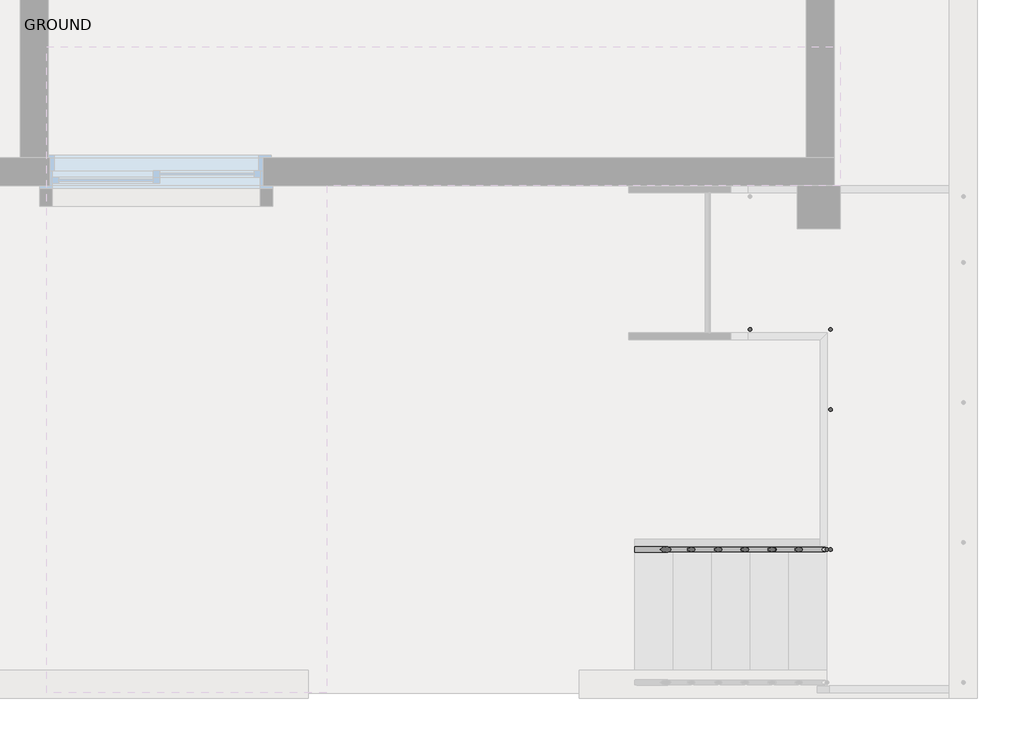
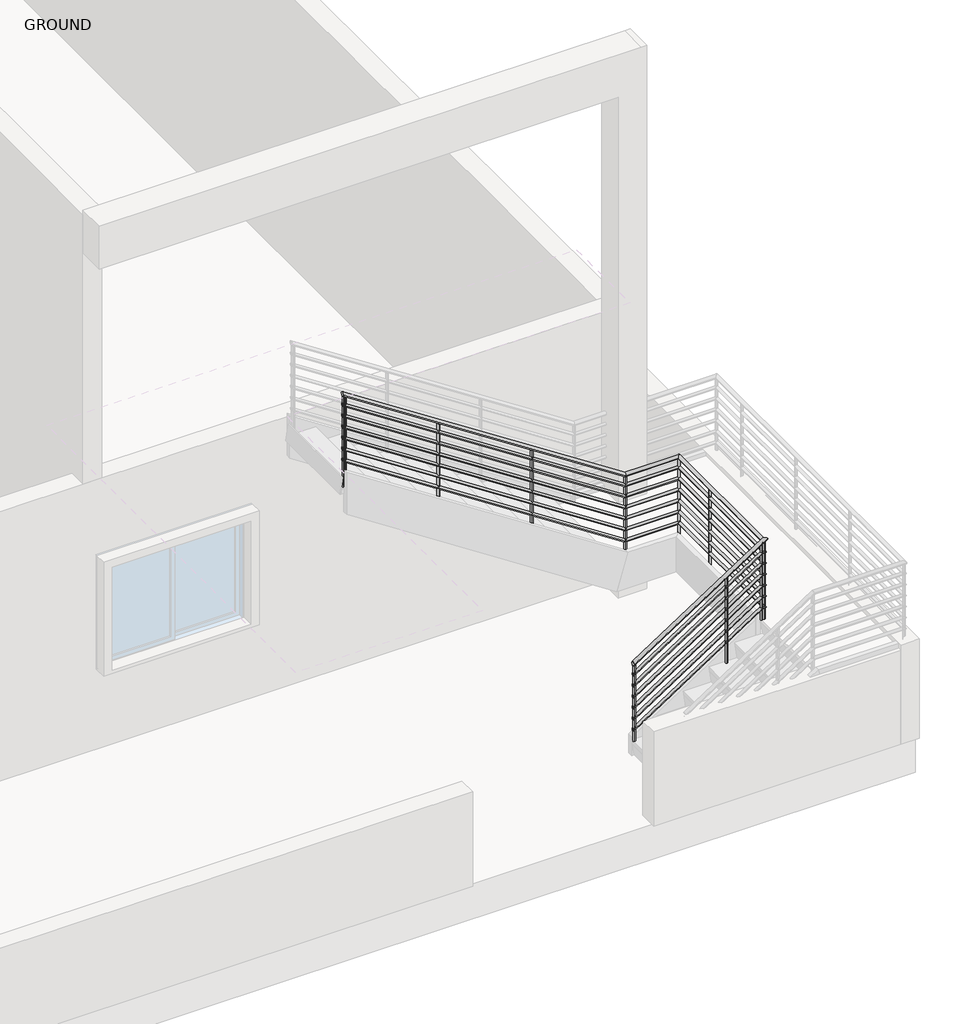
# One storey, part 3 of 4: 1 railing.
"""IFC4 building model written with IfcOpenShell, lengths in millimetres."""

from ifc_helpers import new_model, si_unit, point, frame, frame_2d, origin, place, context, project, spatial, circle_curve, ellipse_curve, trimmed, segment, composite_curve, outline, extrude, element, save
from ifc_brep_helpers import plane_surface, cylinder_surface, advanced_brep

model = new_model("IFC4")

# Units and contexts
model_context = context("Model", 3, world=origin())
ifc_project = project(units=[si_unit("LENGTHUNIT", "METRE", prefix="MILLI")], contexts=[model_context])

# Site, building, storey
site = spatial("IfcSite", under=ifc_project)
building = spatial("IfcBuilding", under=site)
storey = spatial("IfcBuildingStorey", under=building, Name="GROUND", Elevation=0.0)

# Railing
placement = place(None, origin())
element("IfcRailing", 1, ObjectType="900mm Pipe", at=placement, inside=storey, context=model_context, shape_type="SolidModel", body=[
    advanced_brep(
    [(11825.7864069, -2579.127917, 1055.4188073), (11825.7864069, -2539.127917, 1055.4188073), (13253.8631757, -2579.127917, 1986.4943135), (13220.3557578, -2539.127917, 1964.6481938)],
    [
        (0, 1, ellipse_curve(frame((11825.7864069, -2559.127917, 1055.4188073), z_axis=(-1.0, 0.0, 0.0), x_axis=(0.0, 0.0, -1.0)), 23.8753103, 20.0)),
        (1, 0, ellipse_curve(frame((11825.7864069, -2559.127917, 1055.4188073), z_axis=(-1.0, 0.0, 0.0), x_axis=(0.0, 0.0, -1.0)), 23.8753103, 20.0)),
        (2, 3, ellipse_curve(frame((13237.1094668, -2559.127917, 1975.5712536), z_axis=(0.592333060098466, 0.7071067811865425, 0.3861884849583095), x_axis=(-0.5923330600984512, 0.7071067811865527, -0.3861884849583129)), 28.2842712, 20.0)),
        (3, 2, ellipse_curve(frame((13237.1094668, -2559.127917, 1975.5712536), z_axis=(0.592333060098466, 0.7071067811865425, 0.3861884849583095), x_axis=(-0.5923330600984512, 0.7071067811865527, -0.3861884849583129)), 28.2842712, 20.0)),
        (0, 2),
        (3, 1),
    ],
    [
        plane_surface(frame((11825.7864069, -2559.127917, 1079.2941176), z_axis=(-1.0, 0.0, 0.0), x_axis=(0.0, 1.0, 0.0))),
        plane_surface(frame((13226.1864069, -2559.127917, 1992.3249626), z_axis=(0.592333060098466, 0.7071067811865425, 0.3861884849583095), x_axis=(0.8056932083084648, -0.5198538590091285, -0.2839197410518156))),
        cylinder_surface(frame((11836.7094668, -2559.127917, 1062.5404087), z_axis=(-0.8376854470331978, 0.0, -0.5461529930603618), x_axis=(0.0, 1.0, 0.0)), 20.0),
    ],
    [
        (0, [[1, 2]]),
        (1, [[3, 4]]),
        (2, [[-1, 5, -4, 6]]),
        (2, [[-2, -6, -3, -5]]),
    ],
),
    advanced_brep(
    [(13246.1864069, -2564.9585661, 1955.7647059), (13206.1864069, -2531.4511482, 1955.7647059), (13246.1864069, -966.5101069, 1955.7647059), (13206.1864069, -1006.5101069, 1955.7647059), (12644.8424844, -966.5101069, 1955.7647059), (12644.8424844, -1006.5101069, 1955.7647059), (9625.7864069, -966.5101069, 3924.1246897), (9625.7864069, -1006.5101069, 3924.1246897)],
    [
        (0, 1, ellipse_curve(frame((13226.1864069, -2548.2048572, 1955.7647059), z_axis=(-0.592333060098466, -0.7071067811865425, -0.3861884849583095), x_axis=(0.5923330600984515, -0.7071067811865525, 0.3861884849583132)), 28.2842712, 20.0)),
        (1, 0, ellipse_curve(frame((13226.1864069, -2548.2048572, 1955.7647059), z_axis=(-0.592333060098466, -0.7071067811865425, -0.3861884849583095), x_axis=(0.5923330600984515, -0.7071067811865525, 0.3861884849583132)), 28.2842712, 20.0)),
        (0, 2),
        (2, 3, ellipse_curve(frame((13226.1864069, -986.5101069, 1955.7647059), z_axis=(0.7071067811865414, -0.7071067811865537, 0.0), x_axis=(-0.7071067811865537, -0.7071067811865414, 0.0)), 28.2842712, 20.0)),
        (3, 1),
        (3, 2, ellipse_curve(frame((13226.1864069, -986.5101069, 1955.7647059), z_axis=(0.7071067811865414, -0.7071067811865537, 0.0), x_axis=(-0.7071067811865537, -0.7071067811865414, 0.0)), 28.2842712, 20.0)),
        (2, 4),
        (4, 5, ellipse_curve(frame((12644.8424844, -986.5101069, 1955.7647059), z_axis=(0.958562842758157, 0.0, -0.28488116203673575), x_axis=(0.2848811620367357, 0.0, 0.958562842758157)), 20.8645684, 20.0)),
        (5, 3),
        (5, 4, ellipse_curve(frame((12644.8424844, -986.5101069, 1955.7647059), z_axis=(0.958562842758157, 0.0, -0.28488116203673575), x_axis=(0.2848811620367357, 0.0, 0.958562842758157)), 20.8645684, 20.0)),
        (6, 7, ellipse_curve(frame((9625.7864069, -986.5101069, 3924.1246897), z_axis=(-1.0, 0.0, 0.0), x_axis=(0.0, 0.0, -1.0)), 23.8753103, 20.0)),
        (7, 6, ellipse_curve(frame((9625.7864069, -986.5101069, 3924.1246897), z_axis=(-1.0, 0.0, 0.0), x_axis=(0.0, 0.0, -1.0)), 23.8753103, 20.0)),
        (4, 6),
        (7, 5),
    ],
    [
        plane_surface(frame((13226.1864069, -2559.127917, 1975.7647059), z_axis=(-0.592333060098466, -0.7071067811865425, -0.3861884849583095), x_axis=(0.8056932083084648, -0.5198538590091285, -0.2839197410518156))),
        cylinder_surface(frame((13226.1864069, -2559.127917, 1955.7647059), z_axis=(0.0, -1.0, 0.0), x_axis=(-1.0, 0.0, 0.0)), 20.0),
        cylinder_surface(frame((13226.1864069, -986.5101069, 1955.7647059), z_axis=(1.0, 0.0, 0.0), x_axis=(0.0, -1.0, 0.0)), 20.0),
        plane_surface(frame((9625.7864069, -986.5101069, 3948.0), z_axis=(-1.0, 0.0, 0.0), x_axis=(0.0, -1.0, 0.0))),
        cylinder_surface(frame((12639.863347, -986.5101069, 1959.0109969), z_axis=(0.8376854470331982, 0.0, -0.5461529930603611), x_axis=(0.0, -1.0, 0.0)), 20.0),
    ],
    [
        (0, [[1, 2]]),
        (1, [[-1, 3, 4, 5]]),
        (1, [[-2, -5, 6, -3]]),
        (2, [[-4, 7, 8, 9]]),
        (2, [[-6, -9, 10, -7]]),
        (3, [[11, 12]]),
        (4, [[-8, 13, -12, 14]]),
        (4, [[-10, -14, -11, -13]]),
    ],
),
    advanced_brep(
    [(11825.7864069, -2574.127917, 936.3876349), (11825.7864069, -2544.127917, 936.3876349), (13205.2443488, -2574.127917, 1835.7647059), (13205.2443488, -2544.127917, 1835.7647059), (13241.1864069, -2574.127917, 1835.7647059), (13211.1864069, -2544.127917, 1835.7647059), (13241.1864069, -971.5101069, 1835.7647059), (13211.1864069, -1001.5101069, 1835.7647059), (12646.328465, -971.5101069, 1835.7647059), (12646.328465, -1001.5101069, 1835.7647059), (9625.7864069, -971.5101069, 3805.0935173), (9625.7864069, -1001.5101069, 3805.0935173)],
    [
        (0, 1, ellipse_curve(frame((11825.7864069, -2559.127917, 936.3876349), z_axis=(-1.0, 0.0, 0.0), x_axis=(0.0, 0.0, -1.0)), 17.9064827, 15.0)),
        (1, 0, ellipse_curve(frame((11825.7864069, -2559.127917, 936.3876349), z_axis=(-1.0, 0.0, 0.0), x_axis=(0.0, 0.0, -1.0)), 17.9064827, 15.0)),
        (0, 2),
        (2, 3, ellipse_curve(frame((13205.2443488, -2559.127917, 1835.7647059), z_axis=(-0.9585628427581571, 0.0, -0.2848811620367355), x_axis=(0.2848811620367357, 0.0, -0.9585628427581568)), 15.6484263, 15.0)),
        (3, 1),
        (3, 2, ellipse_curve(frame((13205.2443488, -2559.127917, 1835.7647059), z_axis=(-0.9585628427581571, 0.0, -0.2848811620367355), x_axis=(0.2848811620367357, 0.0, -0.9585628427581568)), 15.6484263, 15.0)),
        (2, 4),
        (4, 5, ellipse_curve(frame((13226.1864069, -2559.127917, 1835.7647059), z_axis=(-0.7071067811865537, -0.7071067811865414, 0.0), x_axis=(-0.7071067811865414, 0.7071067811865537, 0.0)), 21.2132034, 15.0)),
        (5, 3),
        (5, 4, ellipse_curve(frame((13226.1864069, -2559.127917, 1835.7647059), z_axis=(-0.7071067811865537, -0.7071067811865414, 0.0), x_axis=(-0.7071067811865414, 0.7071067811865537, 0.0)), 21.2132034, 15.0)),
        (4, 6),
        (6, 7, ellipse_curve(frame((13226.1864069, -986.5101069, 1835.7647059), z_axis=(0.7071067811865414, -0.7071067811865537, 0.0), x_axis=(-0.7071067811865538, -0.7071067811865414, 0.0)), 21.2132034, 15.0)),
        (7, 5),
        (7, 6, ellipse_curve(frame((13226.1864069, -986.5101069, 1835.7647059), z_axis=(0.7071067811865414, -0.7071067811865537, 0.0), x_axis=(-0.7071067811865538, -0.7071067811865414, 0.0)), 21.2132034, 15.0)),
        (6, 8),
        (8, 9, ellipse_curve(frame((12646.328465, -986.5101069, 1835.7647059), z_axis=(0.958562842758157, 0.0, -0.2848811620367359), x_axis=(0.28488116203673564, 0.0, 0.958562842758157)), 15.6484263, 15.0)),
        (9, 7),
        (9, 8, ellipse_curve(frame((12646.328465, -986.5101069, 1835.7647059), z_axis=(0.958562842758157, 0.0, -0.2848811620367359), x_axis=(0.28488116203673564, 0.0, 0.958562842758157)), 15.6484263, 15.0)),
        (10, 11, ellipse_curve(frame((9625.7864069, -986.5101069, 3805.0935173), z_axis=(-1.0, 0.0, 0.0), x_axis=(0.0, 0.0, -1.0)), 17.9064827, 15.0)),
        (11, 10, ellipse_curve(frame((9625.7864069, -986.5101069, 3805.0935173), z_axis=(-1.0, 0.0, 0.0), x_axis=(0.0, 0.0, -1.0)), 17.9064827, 15.0)),
        (8, 10),
        (11, 9),
    ],
    [
        plane_surface(frame((11825.7864069, -2559.127917, 954.2941176), z_axis=(-1.0, 0.0, 0.0), x_axis=(0.0, 1.0, 0.0))),
        cylinder_surface(frame((11833.9787018, -2559.127917, 941.7288359), z_axis=(-0.8376854470331986, 0.0, -0.5461529930603606), x_axis=(0.0, 1.0, 0.0)), 15.0),
        cylinder_surface(frame((13200.7864069, -2559.127917, 1835.7647059), z_axis=(-1.0, 0.0, 0.0), x_axis=(0.0, 1.0, 0.0)), 15.0),
        cylinder_surface(frame((13226.1864069, -2559.127917, 1835.7647059), z_axis=(0.0, -1.0, 0.0), x_axis=(-1.0, 0.0, 0.0)), 15.0),
        cylinder_surface(frame((13226.1864069, -986.5101069, 1835.7647059), z_axis=(1.0, 0.0, 0.0), x_axis=(0.0, -1.0, 0.0)), 15.0),
        plane_surface(frame((9625.7864069, -986.5101069, 3823.0), z_axis=(-1.0, 0.0, 0.0), x_axis=(0.0, -1.0, 0.0))),
        cylinder_surface(frame((12642.594112, -986.5101069, 1838.1994242), z_axis=(0.8376854470331982, 0.0, -0.5461529930603612), x_axis=(0.0, -1.0, 0.0)), 15.0),
    ],
    [
        (0, [[1, 2]]),
        (1, [[-1, 3, 4, 5]]),
        (1, [[-2, -5, 6, -3]]),
        (2, [[-4, 7, 8, 9]]),
        (2, [[-6, -9, 10, -7]]),
        (3, [[-8, 11, 12, 13]]),
        (3, [[-10, -13, 14, -11]]),
        (4, [[-12, 15, 16, 17]]),
        (4, [[-14, -17, 18, -15]]),
        (5, [[19, 20]]),
        (6, [[-16, 21, -20, 22]]),
        (6, [[-18, -22, -19, -21]]),
    ],
),
    advanced_brep(
    [(11825.7864069, -2574.127917, 811.3876349), (11825.7864069, -2544.127917, 811.3876349), (13205.2443488, -2574.127917, 1710.7647059), (13205.2443488, -2544.127917, 1710.7647059), (13241.1864069, -2574.127917, 1710.7647059), (13211.1864069, -2544.127917, 1710.7647059), (13241.1864069, -971.5101069, 1710.7647059), (13211.1864069, -1001.5101069, 1710.7647059), (12646.328465, -971.5101069, 1710.7647059), (12646.328465, -1001.5101069, 1710.7647059), (9625.7864069, -971.5101069, 3680.0935173), (9625.7864069, -1001.5101069, 3680.0935173)],
    [
        (0, 1, ellipse_curve(frame((11825.7864069, -2559.127917, 811.3876349), z_axis=(-1.0, 0.0, 0.0), x_axis=(0.0, 0.0, -1.0)), 17.9064827, 15.0)),
        (1, 0, ellipse_curve(frame((11825.7864069, -2559.127917, 811.3876349), z_axis=(-1.0, 0.0, 0.0), x_axis=(0.0, 0.0, -1.0)), 17.9064827, 15.0)),
        (0, 2),
        (2, 3, ellipse_curve(frame((13205.2443488, -2559.127917, 1710.7647059), z_axis=(-0.9585628427581571, 0.0, -0.2848811620367356), x_axis=(0.2848811620367359, 0.0, -0.958562842758157)), 15.6484263, 15.0)),
        (3, 1),
        (3, 2, ellipse_curve(frame((13205.2443488, -2559.127917, 1710.7647059), z_axis=(-0.9585628427581571, 0.0, -0.2848811620367356), x_axis=(0.2848811620367359, 0.0, -0.958562842758157)), 15.6484263, 15.0)),
        (2, 4),
        (4, 5, ellipse_curve(frame((13226.1864069, -2559.127917, 1710.7647059), z_axis=(-0.7071067811865537, -0.7071067811865414, 0.0), x_axis=(-0.7071067811865414, 0.7071067811865537, 0.0)), 21.2132034, 15.0)),
        (5, 3),
        (5, 4, ellipse_curve(frame((13226.1864069, -2559.127917, 1710.7647059), z_axis=(-0.7071067811865537, -0.7071067811865414, 0.0), x_axis=(-0.7071067811865414, 0.7071067811865537, 0.0)), 21.2132034, 15.0)),
        (4, 6),
        (6, 7, ellipse_curve(frame((13226.1864069, -986.5101069, 1710.7647059), z_axis=(0.7071067811865414, -0.7071067811865537, 0.0), x_axis=(-0.7071067811865538, -0.7071067811865414, 0.0)), 21.2132034, 15.0)),
        (7, 5),
        (7, 6, ellipse_curve(frame((13226.1864069, -986.5101069, 1710.7647059), z_axis=(0.7071067811865414, -0.7071067811865537, 0.0), x_axis=(-0.7071067811865538, -0.7071067811865414, 0.0)), 21.2132034, 15.0)),
        (6, 8),
        (8, 9, ellipse_curve(frame((12646.328465, -986.5101069, 1710.7647059), z_axis=(0.958562842758157, 0.0, -0.28488116203673575), x_axis=(0.2848811620367357, 0.0, 0.958562842758157)), 15.6484263, 15.0)),
        (9, 7),
        (9, 8, ellipse_curve(frame((12646.328465, -986.5101069, 1710.7647059), z_axis=(0.958562842758157, 0.0, -0.28488116203673575), x_axis=(0.2848811620367357, 0.0, 0.958562842758157)), 15.6484263, 15.0)),
        (10, 11, ellipse_curve(frame((9625.7864069, -986.5101069, 3680.0935173), z_axis=(-1.0, 0.0, 0.0), x_axis=(0.0, 0.0, -1.0)), 17.9064827, 15.0)),
        (11, 10, ellipse_curve(frame((9625.7864069, -986.5101069, 3680.0935173), z_axis=(-1.0, 0.0, 0.0), x_axis=(0.0, 0.0, -1.0)), 17.9064827, 15.0)),
        (8, 10),
        (11, 9),
    ],
    [
        plane_surface(frame((11825.7864069, -2559.127917, 829.2941176), z_axis=(-1.0, 0.0, 0.0), x_axis=(0.0, 1.0, 0.0))),
        cylinder_surface(frame((11833.9787018, -2559.127917, 816.7288359), z_axis=(-0.8376854470331985, 0.0, -0.5461529930603608), x_axis=(0.0, 1.0, 0.0)), 15.0),
        cylinder_surface(frame((13200.7864069, -2559.127917, 1710.7647059), z_axis=(-1.0, 0.0, 0.0), x_axis=(0.0, 1.0, 0.0)), 15.0),
        cylinder_surface(frame((13226.1864069, -2559.127917, 1710.7647059), z_axis=(0.0, -1.0, 0.0), x_axis=(-1.0, 0.0, 0.0)), 15.0),
        cylinder_surface(frame((13226.1864069, -986.5101069, 1710.7647059), z_axis=(1.0, 0.0, 0.0), x_axis=(0.0, -1.0, 0.0)), 15.0),
        plane_surface(frame((9625.7864069, -986.5101069, 3698.0), z_axis=(-1.0, 0.0, 0.0), x_axis=(0.0, -1.0, 0.0))),
        cylinder_surface(frame((12642.594112, -986.5101069, 1713.1994242), z_axis=(0.8376854470331982, 0.0, -0.5461529930603611), x_axis=(0.0, -1.0, 0.0)), 15.0),
    ],
    [
        (0, [[1, 2]]),
        (1, [[-1, 3, 4, 5]]),
        (1, [[-2, -5, 6, -3]]),
        (2, [[-4, 7, 8, 9]]),
        (2, [[-6, -9, 10, -7]]),
        (3, [[-8, 11, 12, 13]]),
        (3, [[-10, -13, 14, -11]]),
        (4, [[-12, 15, 16, 17]]),
        (4, [[-14, -17, 18, -15]]),
        (5, [[19, 20]]),
        (6, [[-16, 21, -20, 22]]),
        (6, [[-18, -22, -19, -21]]),
    ],
),
    advanced_brep(
    [(11825.7864069, -2574.127917, 686.3876349), (11825.7864069, -2544.127917, 686.3876349), (13205.2443488, -2574.127917, 1585.7647059), (13205.2443488, -2544.127917, 1585.7647059), (13241.1864069, -2574.127917, 1585.7647059), (13211.1864069, -2544.127917, 1585.7647059), (13241.1864069, -971.5101069, 1585.7647059), (13211.1864069, -1001.5101069, 1585.7647059), (12646.328465, -971.5101069, 1585.7647059), (12646.328465, -1001.5101069, 1585.7647059), (9625.7864069, -971.5101069, 3555.0935173), (9625.7864069, -1001.5101069, 3555.0935173)],
    [
        (0, 1, ellipse_curve(frame((11825.7864069, -2559.127917, 686.3876349), z_axis=(-1.0, 0.0, 0.0), x_axis=(0.0, 0.0, -1.0)), 17.9064827, 15.0)),
        (1, 0, ellipse_curve(frame((11825.7864069, -2559.127917, 686.3876349), z_axis=(-1.0, 0.0, 0.0), x_axis=(0.0, 0.0, -1.0)), 17.9064827, 15.0)),
        (0, 2),
        (2, 3, ellipse_curve(frame((13205.2443488, -2559.127917, 1585.7647059), z_axis=(-0.9585628427581571, 0.0, -0.2848811620367355), x_axis=(0.2848811620367357, 0.0, -0.9585628427581568)), 15.6484263, 15.0)),
        (3, 1),
        (3, 2, ellipse_curve(frame((13205.2443488, -2559.127917, 1585.7647059), z_axis=(-0.9585628427581571, 0.0, -0.2848811620367355), x_axis=(0.2848811620367357, 0.0, -0.9585628427581568)), 15.6484263, 15.0)),
        (2, 4),
        (4, 5, ellipse_curve(frame((13226.1864069, -2559.127917, 1585.7647059), z_axis=(-0.7071067811865537, -0.7071067811865414, 0.0), x_axis=(-0.7071067811865414, 0.7071067811865537, 0.0)), 21.2132034, 15.0)),
        (5, 3),
        (5, 4, ellipse_curve(frame((13226.1864069, -2559.127917, 1585.7647059), z_axis=(-0.7071067811865537, -0.7071067811865414, 0.0), x_axis=(-0.7071067811865414, 0.7071067811865537, 0.0)), 21.2132034, 15.0)),
        (4, 6),
        (6, 7, ellipse_curve(frame((13226.1864069, -986.5101069, 1585.7647059), z_axis=(0.7071067811865414, -0.7071067811865537, 0.0), x_axis=(-0.7071067811865538, -0.7071067811865414, 0.0)), 21.2132034, 15.0)),
        (7, 5),
        (7, 6, ellipse_curve(frame((13226.1864069, -986.5101069, 1585.7647059), z_axis=(0.7071067811865414, -0.7071067811865537, 0.0), x_axis=(-0.7071067811865538, -0.7071067811865414, 0.0)), 21.2132034, 15.0)),
        (6, 8),
        (8, 9, ellipse_curve(frame((12646.328465, -986.5101069, 1585.7647059), z_axis=(0.958562842758157, 0.0, -0.28488116203673575), x_axis=(0.2848811620367358, 0.0, 0.9585628427581571)), 15.6484263, 15.0)),
        (9, 7),
        (9, 8, ellipse_curve(frame((12646.328465, -986.5101069, 1585.7647059), z_axis=(0.958562842758157, 0.0, -0.28488116203673575), x_axis=(0.2848811620367358, 0.0, 0.9585628427581571)), 15.6484263, 15.0)),
        (10, 11, ellipse_curve(frame((9625.7864069, -986.5101069, 3555.0935173), z_axis=(-1.0, 0.0, 0.0), x_axis=(0.0, 0.0, -1.0)), 17.9064827, 15.0)),
        (11, 10, ellipse_curve(frame((9625.7864069, -986.5101069, 3555.0935173), z_axis=(-1.0, 0.0, 0.0), x_axis=(0.0, 0.0, -1.0)), 17.9064827, 15.0)),
        (8, 10),
        (11, 9),
    ],
    [
        plane_surface(frame((11825.7864069, -2559.127917, 704.2941176), z_axis=(-1.0, 0.0, 0.0), x_axis=(0.0, 1.0, 0.0))),
        cylinder_surface(frame((11833.9787018, -2559.127917, 691.7288359), z_axis=(-0.8376854470331986, 0.0, -0.5461529930603606), x_axis=(0.0, 1.0, 0.0)), 15.0),
        cylinder_surface(frame((13200.7864069, -2559.127917, 1585.7647059), z_axis=(-1.0, 0.0, 0.0), x_axis=(0.0, 1.0, 0.0)), 15.0),
        cylinder_surface(frame((13226.1864069, -2559.127917, 1585.7647059), z_axis=(0.0, -1.0, 0.0), x_axis=(-1.0, 0.0, 0.0)), 15.0),
        cylinder_surface(frame((13226.1864069, -986.5101069, 1585.7647059), z_axis=(1.0, 0.0, 0.0), x_axis=(0.0, -1.0, 0.0)), 15.0),
        plane_surface(frame((9625.7864069, -986.5101069, 3573.0), z_axis=(-1.0, 0.0, 0.0), x_axis=(0.0, -1.0, 0.0))),
        cylinder_surface(frame((12642.594112, -986.5101069, 1588.1994242), z_axis=(0.8376854470331982, 0.0, -0.546152993060361), x_axis=(0.0, -1.0, 0.0)), 15.0),
    ],
    [
        (0, [[1, 2]]),
        (1, [[-1, 3, 4, 5]]),
        (1, [[-2, -5, 6, -3]]),
        (2, [[-4, 7, 8, 9]]),
        (2, [[-6, -9, 10, -7]]),
        (3, [[-8, 11, 12, 13]]),
        (3, [[-10, -13, 14, -11]]),
        (4, [[-12, 15, 16, 17]]),
        (4, [[-14, -17, 18, -15]]),
        (5, [[19, 20]]),
        (6, [[-16, 21, -20, 22]]),
        (6, [[-18, -22, -19, -21]]),
    ],
),
    advanced_brep(
    [(11825.7864069, -2574.127917, 561.3876349), (11825.7864069, -2544.127917, 561.3876349), (13205.2443488, -2574.127917, 1460.7647059), (13205.2443488, -2544.127917, 1460.7647059), (13241.1864069, -2574.127917, 1460.7647059), (13211.1864069, -2544.127917, 1460.7647059), (13241.1864069, -971.5101069, 1460.7647059), (13211.1864069, -1001.5101069, 1460.7647059), (12646.328465, -971.5101069, 1460.7647059), (12646.328465, -1001.5101069, 1460.7647059), (9625.7864069, -971.5101069, 3430.0935173), (9625.7864069, -1001.5101069, 3430.0935173)],
    [
        (0, 1, ellipse_curve(frame((11825.7864069, -2559.127917, 561.3876349), z_axis=(-1.0, 0.0, 0.0), x_axis=(0.0, 0.0, -1.0)), 17.9064827, 15.0)),
        (1, 0, ellipse_curve(frame((11825.7864069, -2559.127917, 561.3876349), z_axis=(-1.0, 0.0, 0.0), x_axis=(0.0, 0.0, -1.0)), 17.9064827, 15.0)),
        (0, 2),
        (2, 3, ellipse_curve(frame((13205.2443488, -2559.127917, 1460.7647059), z_axis=(-0.9585628427581571, 0.0, -0.2848811620367356), x_axis=(0.2848811620367359, 0.0, -0.958562842758157)), 15.6484263, 15.0)),
        (3, 1),
        (3, 2, ellipse_curve(frame((13205.2443488, -2559.127917, 1460.7647059), z_axis=(-0.9585628427581571, 0.0, -0.2848811620367356), x_axis=(0.2848811620367359, 0.0, -0.958562842758157)), 15.6484263, 15.0)),
        (2, 4),
        (4, 5, ellipse_curve(frame((13226.1864069, -2559.127917, 1460.7647059), z_axis=(-0.7071067811865537, -0.7071067811865414, 0.0), x_axis=(-0.7071067811865414, 0.7071067811865537, 0.0)), 21.2132034, 15.0)),
        (5, 3),
        (5, 4, ellipse_curve(frame((13226.1864069, -2559.127917, 1460.7647059), z_axis=(-0.7071067811865537, -0.7071067811865414, 0.0), x_axis=(-0.7071067811865414, 0.7071067811865537, 0.0)), 21.2132034, 15.0)),
        (4, 6),
        (6, 7, ellipse_curve(frame((13226.1864069, -986.5101069, 1460.7647059), z_axis=(0.7071067811865414, -0.7071067811865537, 0.0), x_axis=(-0.7071067811865538, -0.7071067811865414, 0.0)), 21.2132034, 15.0)),
        (7, 5),
        (7, 6, ellipse_curve(frame((13226.1864069, -986.5101069, 1460.7647059), z_axis=(0.7071067811865414, -0.7071067811865537, 0.0), x_axis=(-0.7071067811865538, -0.7071067811865414, 0.0)), 21.2132034, 15.0)),
        (6, 8),
        (8, 9, ellipse_curve(frame((12646.328465, -986.5101069, 1460.7647059), z_axis=(0.958562842758157, 0.0, -0.28488116203673575), x_axis=(0.2848811620367357, 0.0, 0.958562842758157)), 15.6484263, 15.0)),
        (9, 7),
        (9, 8, ellipse_curve(frame((12646.328465, -986.5101069, 1460.7647059), z_axis=(0.958562842758157, 0.0, -0.28488116203673575), x_axis=(0.2848811620367357, 0.0, 0.958562842758157)), 15.6484263, 15.0)),
        (10, 11, ellipse_curve(frame((9625.7864069, -986.5101069, 3430.0935173), z_axis=(-1.0, 0.0, 0.0), x_axis=(0.0, 0.0, -1.0)), 17.9064827, 15.0)),
        (11, 10, ellipse_curve(frame((9625.7864069, -986.5101069, 3430.0935173), z_axis=(-1.0, 0.0, 0.0), x_axis=(0.0, 0.0, -1.0)), 17.9064827, 15.0)),
        (8, 10),
        (11, 9),
    ],
    [
        plane_surface(frame((11825.7864069, -2559.127917, 579.2941176), z_axis=(-1.0, 0.0, 0.0), x_axis=(0.0, 1.0, 0.0))),
        cylinder_surface(frame((11833.9787018, -2559.127917, 566.7288359), z_axis=(-0.8376854470331985, 0.0, -0.5461529930603608), x_axis=(0.0, 1.0, 0.0)), 15.0),
        cylinder_surface(frame((13200.7864069, -2559.127917, 1460.7647059), z_axis=(-1.0, 0.0, 0.0), x_axis=(0.0, 1.0, 0.0)), 15.0),
        cylinder_surface(frame((13226.1864069, -2559.127917, 1460.7647059), z_axis=(0.0, -1.0, 0.0), x_axis=(-1.0, 0.0, 0.0)), 15.0),
        cylinder_surface(frame((13226.1864069, -986.5101069, 1460.7647059), z_axis=(1.0, 0.0, 0.0), x_axis=(0.0, -1.0, 0.0)), 15.0),
        plane_surface(frame((9625.7864069, -986.5101069, 3448.0), z_axis=(-1.0, 0.0, 0.0), x_axis=(0.0, -1.0, 0.0))),
        cylinder_surface(frame((12642.594112, -986.5101069, 1463.1994242), z_axis=(0.8376854470331982, 0.0, -0.5461529930603611), x_axis=(0.0, -1.0, 0.0)), 15.0),
    ],
    [
        (0, [[1, 2]]),
        (1, [[-1, 3, 4, 5]]),
        (1, [[-2, -5, 6, -3]]),
        (2, [[-4, 7, 8, 9]]),
        (2, [[-6, -9, 10, -7]]),
        (3, [[-8, 11, 12, 13]]),
        (3, [[-10, -13, 14, -11]]),
        (4, [[-12, 15, 16, 17]]),
        (4, [[-14, -17, 18, -15]]),
        (5, [[19, 20]]),
        (6, [[-16, 21, -20, 22]]),
        (6, [[-18, -22, -19, -21]]),
    ],
),
    advanced_brep(
    [(11825.7864069, -2574.127917, 436.3876349), (11825.7864069, -2544.127917, 436.3876349), (13205.2443488, -2574.127917, 1335.7647059), (13205.2443488, -2544.127917, 1335.7647059), (13241.1864069, -2574.127917, 1335.7647059), (13211.1864069, -2544.127917, 1335.7647059), (13241.1864069, -971.5101069, 1335.7647059), (13211.1864069, -1001.5101069, 1335.7647059), (12646.328465, -971.5101069, 1335.7647059), (12646.328465, -1001.5101069, 1335.7647059), (9625.7864069, -971.5101069, 3305.0935173), (9625.7864069, -1001.5101069, 3305.0935173)],
    [
        (0, 1, ellipse_curve(frame((11825.7864069, -2559.127917, 436.3876349), z_axis=(-1.0, 0.0, 0.0), x_axis=(0.0, 0.0, -1.0)), 17.9064827, 15.0)),
        (1, 0, ellipse_curve(frame((11825.7864069, -2559.127917, 436.3876349), z_axis=(-1.0, 0.0, 0.0), x_axis=(0.0, 0.0, -1.0)), 17.9064827, 15.0)),
        (0, 2),
        (2, 3, ellipse_curve(frame((13205.2443488, -2559.127917, 1335.7647059), z_axis=(-0.9585628427581571, 0.0, -0.2848811620367355), x_axis=(0.2848811620367357, 0.0, -0.9585628427581568)), 15.6484263, 15.0)),
        (3, 1),
        (3, 2, ellipse_curve(frame((13205.2443488, -2559.127917, 1335.7647059), z_axis=(-0.9585628427581571, 0.0, -0.2848811620367355), x_axis=(0.2848811620367357, 0.0, -0.9585628427581568)), 15.6484263, 15.0)),
        (2, 4),
        (4, 5, ellipse_curve(frame((13226.1864069, -2559.127917, 1335.7647059), z_axis=(-0.7071067811865537, -0.7071067811865414, 0.0), x_axis=(-0.7071067811865414, 0.7071067811865537, 0.0)), 21.2132034, 15.0)),
        (5, 3),
        (5, 4, ellipse_curve(frame((13226.1864069, -2559.127917, 1335.7647059), z_axis=(-0.7071067811865537, -0.7071067811865414, 0.0), x_axis=(-0.7071067811865414, 0.7071067811865537, 0.0)), 21.2132034, 15.0)),
        (4, 6),
        (6, 7, ellipse_curve(frame((13226.1864069, -986.5101069, 1335.7647059), z_axis=(0.7071067811865414, -0.7071067811865537, 0.0), x_axis=(-0.7071067811865538, -0.7071067811865414, 0.0)), 21.2132034, 15.0)),
        (7, 5),
        (7, 6, ellipse_curve(frame((13226.1864069, -986.5101069, 1335.7647059), z_axis=(0.7071067811865414, -0.7071067811865537, 0.0), x_axis=(-0.7071067811865538, -0.7071067811865414, 0.0)), 21.2132034, 15.0)),
        (6, 8),
        (8, 9, ellipse_curve(frame((12646.328465, -986.5101069, 1335.7647059), z_axis=(0.958562842758157, 0.0, -0.2848811620367359), x_axis=(0.28488116203673564, 0.0, 0.958562842758157)), 15.6484263, 15.0)),
        (9, 7),
        (9, 8, ellipse_curve(frame((12646.328465, -986.5101069, 1335.7647059), z_axis=(0.958562842758157, 0.0, -0.2848811620367359), x_axis=(0.28488116203673564, 0.0, 0.958562842758157)), 15.6484263, 15.0)),
        (10, 11, ellipse_curve(frame((9625.7864069, -986.5101069, 3305.0935173), z_axis=(-1.0, 0.0, 0.0), x_axis=(0.0, 0.0, -1.0)), 17.9064827, 15.0)),
        (11, 10, ellipse_curve(frame((9625.7864069, -986.5101069, 3305.0935173), z_axis=(-1.0, 0.0, 0.0), x_axis=(0.0, 0.0, -1.0)), 17.9064827, 15.0)),
        (8, 10),
        (11, 9),
    ],
    [
        plane_surface(frame((11825.7864069, -2559.127917, 454.2941176), z_axis=(-1.0, 0.0, 0.0), x_axis=(0.0, 1.0, 0.0))),
        cylinder_surface(frame((11833.9787018, -2559.127917, 441.7288359), z_axis=(-0.8376854470331986, 0.0, -0.5461529930603606), x_axis=(0.0, 1.0, 0.0)), 15.0),
        cylinder_surface(frame((13200.7864069, -2559.127917, 1335.7647059), z_axis=(-1.0, 0.0, 0.0), x_axis=(0.0, 1.0, 0.0)), 15.0),
        cylinder_surface(frame((13226.1864069, -2559.127917, 1335.7647059), z_axis=(0.0, -1.0, 0.0), x_axis=(-1.0, 0.0, 0.0)), 15.0),
        cylinder_surface(frame((13226.1864069, -986.5101069, 1335.7647059), z_axis=(1.0, 0.0, 0.0), x_axis=(0.0, -1.0, 0.0)), 15.0),
        plane_surface(frame((9625.7864069, -986.5101069, 3323.0), z_axis=(-1.0, 0.0, 0.0), x_axis=(0.0, -1.0, 0.0))),
        cylinder_surface(frame((12642.594112, -986.5101069, 1338.1994242), z_axis=(0.8376854470331982, 0.0, -0.5461529930603612), x_axis=(0.0, -1.0, 0.0)), 15.0),
    ],
    [
        (0, [[1, 2]]),
        (1, [[-1, 3, 4, 5]]),
        (1, [[-2, -5, 6, -3]]),
        (2, [[-4, 7, 8, 9]]),
        (2, [[-6, -9, 10, -7]]),
        (3, [[-8, 11, 12, 13]]),
        (3, [[-10, -13, 14, -11]]),
        (4, [[-12, 15, 16, 17]]),
        (4, [[-14, -17, 18, -15]]),
        (5, [[19, 20]]),
        (6, [[-16, 21, -20, 22]]),
        (6, [[-18, -22, -19, -21]]),
    ],
),
    advanced_brep(
    [(11825.7864069, -2574.127917, 311.3876349), (11825.7864069, -2544.127917, 311.3876349), (13205.2443488, -2574.127917, 1210.7647059), (13205.2443488, -2544.127917, 1210.7647059), (13241.1864069, -2574.127917, 1210.7647059), (13211.1864069, -2544.127917, 1210.7647059), (13241.1864069, -971.5101069, 1210.7647059), (13211.1864069, -1001.5101069, 1210.7647059), (12646.328465, -971.5101069, 1210.7647059), (12646.328465, -1001.5101069, 1210.7647059), (9625.7864069, -971.5101069, 3180.0935173), (9625.7864069, -1001.5101069, 3180.0935173)],
    [
        (0, 1, ellipse_curve(frame((11825.7864069, -2559.127917, 311.3876349), z_axis=(-1.0, 0.0, 0.0), x_axis=(0.0, 0.0, -1.0)), 17.9064827, 15.0)),
        (1, 0, ellipse_curve(frame((11825.7864069, -2559.127917, 311.3876349), z_axis=(-1.0, 0.0, 0.0), x_axis=(0.0, 0.0, -1.0)), 17.9064827, 15.0)),
        (0, 2),
        (2, 3, ellipse_curve(frame((13205.2443488, -2559.127917, 1210.7647059), z_axis=(-0.9585628427581571, 0.0, -0.2848811620367356), x_axis=(0.2848811620367359, 0.0, -0.958562842758157)), 15.6484263, 15.0)),
        (3, 1),
        (3, 2, ellipse_curve(frame((13205.2443488, -2559.127917, 1210.7647059), z_axis=(-0.9585628427581571, 0.0, -0.2848811620367356), x_axis=(0.2848811620367359, 0.0, -0.958562842758157)), 15.6484263, 15.0)),
        (2, 4),
        (4, 5, ellipse_curve(frame((13226.1864069, -2559.127917, 1210.7647059), z_axis=(-0.7071067811865537, -0.7071067811865414, 0.0), x_axis=(-0.7071067811865414, 0.7071067811865537, 0.0)), 21.2132034, 15.0)),
        (5, 3),
        (5, 4, ellipse_curve(frame((13226.1864069, -2559.127917, 1210.7647059), z_axis=(-0.7071067811865537, -0.7071067811865414, 0.0), x_axis=(-0.7071067811865414, 0.7071067811865537, 0.0)), 21.2132034, 15.0)),
        (4, 6),
        (6, 7, ellipse_curve(frame((13226.1864069, -986.5101069, 1210.7647059), z_axis=(0.7071067811865414, -0.7071067811865537, 0.0), x_axis=(-0.7071067811865538, -0.7071067811865414, 0.0)), 21.2132034, 15.0)),
        (7, 5),
        (7, 6, ellipse_curve(frame((13226.1864069, -986.5101069, 1210.7647059), z_axis=(0.7071067811865414, -0.7071067811865537, 0.0), x_axis=(-0.7071067811865538, -0.7071067811865414, 0.0)), 21.2132034, 15.0)),
        (6, 8),
        (8, 9, ellipse_curve(frame((12646.328465, -986.5101069, 1210.7647059), z_axis=(0.958562842758157, 0.0, -0.28488116203673575), x_axis=(0.2848811620367357, 0.0, 0.958562842758157)), 15.6484263, 15.0)),
        (9, 7),
        (9, 8, ellipse_curve(frame((12646.328465, -986.5101069, 1210.7647059), z_axis=(0.958562842758157, 0.0, -0.28488116203673575), x_axis=(0.2848811620367357, 0.0, 0.958562842758157)), 15.6484263, 15.0)),
        (10, 11, ellipse_curve(frame((9625.7864069, -986.5101069, 3180.0935173), z_axis=(-1.0, 0.0, 0.0), x_axis=(0.0, 0.0, -1.0)), 17.9064827, 15.0)),
        (11, 10, ellipse_curve(frame((9625.7864069, -986.5101069, 3180.0935173), z_axis=(-1.0, 0.0, 0.0), x_axis=(0.0, 0.0, -1.0)), 17.9064827, 15.0)),
        (8, 10),
        (11, 9),
    ],
    [
        plane_surface(frame((11825.7864069, -2559.127917, 329.2941176), z_axis=(-1.0, 0.0, 0.0), x_axis=(0.0, 1.0, 0.0))),
        cylinder_surface(frame((11833.9787018, -2559.127917, 316.7288359), z_axis=(-0.8376854470331985, 0.0, -0.5461529930603608), x_axis=(0.0, 1.0, 0.0)), 15.0),
        cylinder_surface(frame((13200.7864069, -2559.127917, 1210.7647059), z_axis=(-1.0, 0.0, 0.0), x_axis=(0.0, 1.0, 0.0)), 15.0),
        cylinder_surface(frame((13226.1864069, -2559.127917, 1210.7647059), z_axis=(0.0, -1.0, 0.0), x_axis=(-1.0, 0.0, 0.0)), 15.0),
        cylinder_surface(frame((13226.1864069, -986.5101069, 1210.7647059), z_axis=(1.0, 0.0, 0.0), x_axis=(0.0, -1.0, 0.0)), 15.0),
        plane_surface(frame((9625.7864069, -986.5101069, 3198.0), z_axis=(-1.0, 0.0, 0.0), x_axis=(0.0, -1.0, 0.0))),
        cylinder_surface(frame((12642.594112, -986.5101069, 1213.1994242), z_axis=(0.8376854470331982, 0.0, -0.5461529930603611), x_axis=(0.0, -1.0, 0.0)), 15.0),
    ],
    [
        (0, [[1, 2]]),
        (1, [[-1, 3, 4, 5]]),
        (1, [[-2, -5, 6, -3]]),
        (2, [[-4, 7, 8, 9]]),
        (2, [[-6, -9, 10, -7]]),
        (3, [[-8, 11, 12, 13]]),
        (3, [[-10, -13, 14, -11]]),
        (4, [[-12, 15, 16, 17]]),
        (4, [[-14, -17, 18, -15]]),
        (5, [[19, 20]]),
        (6, [[-16, 21, -20, 22]]),
        (6, [[-18, -22, -19, -21]]),
    ],
),
    advanced_brep(
    [(9650.7864069, -999.0101069, 3883.9499141), (9650.7864069, -974.0101069, 3883.9499141), (9650.7864069, -974.0101069, 2868.7058824), (9650.7864069, -999.0101069, 2868.7058824)],
    [
        (0, 1, ellipse_curve(frame((9650.7864069, -986.5101069, 3883.9499141), z_axis=(-0.546152993060361, 0.0, -0.8376854470331982), x_axis=(-0.8376854470331982, 0.0, 0.546152993060361)), 14.922069, 12.5)),
        (1, 2),
        (2, 3, circle_curve(frame((9650.7864069, -986.5101069, 2868.7058824), z_axis=(0.0, 0.0, 1.0), x_axis=(0.0, 1.0, 0.0)), 12.5)),
        (3, 0),
        (3, 2, circle_curve(frame((9650.7864069, -986.5101069, 2868.7058824), z_axis=(0.0, 0.0, 1.0), x_axis=(0.0, 1.0, 0.0)), 12.5)),
        (1, 0, ellipse_curve(frame((9650.7864069, -986.5101069, 3883.9499141), z_axis=(-0.546152993060361, 0.0, -0.8376854470331982), x_axis=(-0.8376854470331982, 0.0, 0.546152993060361)), 14.922069, 12.5)),
    ],
    [
        cylinder_surface(frame((9650.7864069, -986.5101069, 2768.7058824), z_axis=(0.0, 0.0, 1.0), x_axis=(0.0, 1.0, 0.0)), 12.5),
        plane_surface(frame((9625.7864069, -961.5101069, 3900.2493794), z_axis=(0.546152993060361, 0.0, 0.8376854470331982), x_axis=(0.0, -1.0, 0.0))),
        plane_surface(frame((9675.7864069, -961.5101069, 2868.7058824), z_axis=(0.0, 0.0, -1.0), x_axis=(0.0, -1.0, 0.0))),
    ],
    [
        (0, [[1, 2, 3, 4]]),
        (0, [[5, -2, 6, -4]]),
        (1, [[-6, -1]]),
        (2, [[-5, -3]]),
    ],
),
    advanced_brep(
    [(10650.7864069, -999.0101069, 3231.9713045), (10650.7864069, -974.0101069, 3231.9713045), (10650.7864069, -974.0101069, 2330.8235294), (10650.7864069, -999.0101069, 2330.8235294)],
    [
        (0, 1, ellipse_curve(frame((10650.7864069, -986.5101069, 3231.9713045), z_axis=(-0.5461529930603595, 0.0, -0.8376854470331992), x_axis=(-0.8376854470331992, 0.0, 0.5461529930603595)), 14.922069, 12.5)),
        (1, 2),
        (2, 3, circle_curve(frame((10650.7864069, -986.5101069, 2330.8235294), z_axis=(0.0, 0.0, 1.0), x_axis=(0.0, 1.0, 0.0)), 12.5)),
        (3, 0),
        (3, 2, circle_curve(frame((10650.7864069, -986.5101069, 2330.8235294), z_axis=(0.0, 0.0, 1.0), x_axis=(0.0, 1.0, 0.0)), 12.5)),
        (1, 0, ellipse_curve(frame((10650.7864069, -986.5101069, 3231.9713045), z_axis=(-0.5461529930603595, 0.0, -0.8376854470331992), x_axis=(-0.8376854470331992, 0.0, 0.5461529930603595)), 14.922069, 12.5)),
    ],
    [
        cylinder_surface(frame((10650.7864069, -986.5101069, 2230.8235294), z_axis=(0.0, 0.0, 1.0), x_axis=(0.0, 1.0, 0.0)), 12.5),
        plane_surface(frame((10625.7864069, -961.5101069, 3248.2707697), z_axis=(0.5461529930603595, 0.0, 0.8376854470331992), x_axis=(0.0, -1.0, 0.0))),
        plane_surface(frame((10675.7864069, -961.5101069, 2330.8235294), z_axis=(0.0, 0.0, -1.0), x_axis=(0.0, -1.0, 0.0))),
    ],
    [
        (0, [[1, 2, 3, 4]]),
        (0, [[5, -2, 6, -4]]),
        (1, [[-6, -1]]),
        (2, [[-5, -3]]),
    ],
),
    advanced_brep(
    [(11650.7864069, -999.0101069, 2579.9926949), (11650.7864069, -974.0101069, 2579.9926949), (11650.7864069, -974.0101069, 1613.6470588), (11650.7864069, -999.0101069, 1613.6470588)],
    [
        (0, 1, ellipse_curve(frame((11650.7864069, -986.5101069, 2579.9926949), z_axis=(-0.5461529930603595, 0.0, -0.8376854470331992), x_axis=(-0.8376854470331992, 0.0, 0.5461529930603595)), 14.922069, 12.5)),
        (1, 2),
        (2, 3, circle_curve(frame((11650.7864069, -986.5101069, 1613.6470588), z_axis=(0.0, 0.0, 1.0), x_axis=(0.0, 1.0, 0.0)), 12.5)),
        (3, 0),
        (3, 2, circle_curve(frame((11650.7864069, -986.5101069, 1613.6470588), z_axis=(0.0, 0.0, 1.0), x_axis=(0.0, 1.0, 0.0)), 12.5)),
        (1, 0, ellipse_curve(frame((11650.7864069, -986.5101069, 2579.9926949), z_axis=(-0.5461529930603595, 0.0, -0.8376854470331992), x_axis=(-0.8376854470331992, 0.0, 0.5461529930603595)), 14.922069, 12.5)),
    ],
    [
        cylinder_surface(frame((11650.7864069, -986.5101069, 1513.6470588), z_axis=(0.0, 0.0, 1.0), x_axis=(0.0, 1.0, 0.0)), 12.5),
        plane_surface(frame((11625.7864069, -961.5101069, 2596.2921601), z_axis=(0.5461529930603595, 0.0, 0.8376854470331992), x_axis=(0.0, -1.0, 0.0))),
        plane_surface(frame((11675.7864069, -961.5101069, 1613.6470588), z_axis=(0.0, 0.0, -1.0), x_axis=(0.0, -1.0, 0.0))),
    ],
    [
        (0, [[1, 2, 3, 4]]),
        (0, [[5, -2, 6, -4]]),
        (1, [[-6, -1]]),
        (2, [[-5, -3]]),
    ],
),
    extrude(outline(composite_curve([segment(trimmed(circle_curve(frame_2d((13226.1864069, -1559.127917)), 12.5), [point((13238.6864069, -1559.127917))], [point((13213.6864069, -1559.127917))], False, "CARTESIAN"), True, "CONTINUOUS"), segment(trimmed(circle_curve(frame_2d((13226.1864069, -1559.127917)), 12.5), [point((13213.6864069, -1559.127917))], [point((13238.6864069, -1559.127917))], False, "CARTESIAN"), True, "CONTINUOUS")], self_intersect=False)), frame((0.0, 0.0, 1075.7647059), z_axis=(0.0, 0.0, 1.0), x_axis=(1.0, 0.0, 0.0)), (0.0, 0.0, 1.0), 860.0),
    advanced_brep(
    [(12825.7864069, -2546.627917, 1683.5221066), (12825.7864069, -2571.627917, 1683.5221066), (12825.7864069, -2571.627917, 717.1764706), (12825.7864069, -2546.627917, 717.1764706)],
    [
        (0, 1, ellipse_curve(frame((12825.7864069, -2559.127917, 1683.5221066), z_axis=(0.5461529930603595, 0.0, -0.8376854470331992), x_axis=(0.8376854470331992, 0.0, 0.5461529930603595)), 14.922069, 12.5)),
        (1, 2),
        (2, 3, circle_curve(frame((12825.7864069, -2559.127917, 717.1764706), z_axis=(0.0, 0.0, 1.0), x_axis=(0.0, -1.0, 0.0)), 12.5)),
        (3, 0),
        (3, 2, circle_curve(frame((12825.7864069, -2559.127917, 717.1764706), z_axis=(0.0, 0.0, 1.0), x_axis=(0.0, -1.0, 0.0)), 12.5)),
        (1, 0, ellipse_curve(frame((12825.7864069, -2559.127917, 1683.5221066), z_axis=(0.5461529930603595, 0.0, -0.8376854470331992), x_axis=(0.8376854470331992, 0.0, 0.5461529930603595)), 14.922069, 12.5)),
    ],
    [
        cylinder_surface(frame((12825.7864069, -2559.127917, 617.1764706), z_axis=(0.0, 0.0, 1.0), x_axis=(0.0, -1.0, 0.0)), 12.5),
        plane_surface(frame((12850.7864069, -2584.127917, 1699.8215719), z_axis=(-0.5461529930603595, 0.0, 0.8376854470331992), x_axis=(0.0, 1.0, 0.0))),
        plane_surface(frame((12800.7864069, -2584.127917, 717.1764706), z_axis=(0.0, 0.0, -1.0), x_axis=(0.0, 1.0, 0.0))),
    ],
    [
        (0, [[1, 2, 3, 4]]),
        (0, [[5, -2, 6, -4]]),
        (1, [[-6, -1]]),
        (2, [[-5, -3]]),
    ],
),
    extrude(outline(composite_curve([segment(trimmed(circle_curve(frame_2d((12650.7864069, -986.5101069)), 12.5), [point((12650.7864069, -974.0101069))], [point((12650.7864069, -999.0101069))], False, "CARTESIAN"), True, "CONTINUOUS"), segment(trimmed(circle_curve(frame_2d((12650.7864069, -986.5101069)), 12.5), [point((12650.7864069, -999.0101069))], [point((12650.7864069, -974.0101069))], False, "CARTESIAN"), True, "CONTINUOUS")], self_intersect=False)), frame((0.0, 0.0, 1075.7647059), z_axis=(0.0, 0.0, 1.0), x_axis=(1.0, 0.0, 0.0)), (0.0, 0.0, 1.0), 860.0),
    extrude(outline(composite_curve([segment(trimmed(circle_curve(frame_2d((13226.1864069, -986.5101069)), 12.5), [point((13238.6864069, -986.5101069))], [point((13213.6864069, -986.5101069))], False, "CARTESIAN"), True, "CONTINUOUS"), segment(trimmed(circle_curve(frame_2d((13226.1864069, -986.5101069)), 12.5), [point((13213.6864069, -986.5101069))], [point((13238.6864069, -986.5101069))], False, "CARTESIAN"), True, "CONTINUOUS")], self_intersect=False)), frame((0.0, 0.0, 1075.7647059), z_axis=(0.0, 0.0, 1.0), x_axis=(1.0, 0.0, 0.0)), (0.0, 0.0, 1.0), 860.0),
    advanced_brep(
    [(13226.1864069, -2546.627917, 1944.5743419), (13226.1864069, -2571.627917, 1944.5743419), (13226.1864069, -2571.627917, 1075.7647059), (13226.1864069, -2546.627917, 1075.7647059)],
    [
        (0, 1, ellipse_curve(frame((13226.1864069, -2559.127917, 1944.5743419), z_axis=(0.5461529930603595, 0.0, -0.8376854470331992), x_axis=(0.8376854470331992, 0.0, 0.5461529930603595)), 14.922069, 12.5)),
        (1, 2),
        (2, 3, circle_curve(frame((13226.1864069, -2559.127917, 1075.7647059), z_axis=(0.0, 0.0, 1.0), x_axis=(0.0, -1.0, 0.0)), 12.5)),
        (3, 0),
        (3, 2, circle_curve(frame((13226.1864069, -2559.127917, 1075.7647059), z_axis=(0.0, 0.0, 1.0), x_axis=(0.0, -1.0, 0.0)), 12.5)),
        (1, 0, ellipse_curve(frame((13226.1864069, -2559.127917, 1944.5743419), z_axis=(0.5461529930603595, 0.0, -0.8376854470331992), x_axis=(0.8376854470331992, 0.0, 0.5461529930603595)), 14.922069, 12.5)),
    ],
    [
        cylinder_surface(frame((13226.1864069, -2559.127917, 975.7647059), z_axis=(0.0, 0.0, 1.0), x_axis=(0.0, -1.0, 0.0)), 12.5),
        plane_surface(frame((13251.1864069, -2584.127917, 1960.8738072), z_axis=(-0.5461529930603595, 0.0, 0.8376854470331992), x_axis=(0.0, 1.0, 0.0))),
        plane_surface(frame((13201.1864069, -2584.127917, 1075.7647059), z_axis=(0.0, 0.0, -1.0), x_axis=(0.0, 1.0, 0.0))),
    ],
    [
        (0, [[1, 2, 3, 4]]),
        (0, [[5, -2, 6, -4]]),
        (1, [[-6, -1]]),
        (2, [[-5, -3]]),
    ],
),
    advanced_brep(
    [(13200.7864069, -2546.627917, 1928.0140852), (13200.7864069, -2571.627917, 1928.0140852), (13200.7864069, -2571.627917, 1075.7647059), (13200.7864069, -2546.627917, 1075.7647059)],
    [
        (0, 1, ellipse_curve(frame((13200.7864069, -2559.127917, 1928.0140852), z_axis=(0.546152993060361, 0.0, -0.8376854470331982), x_axis=(0.8376854470331982, 0.0, 0.546152993060361)), 14.922069, 12.5)),
        (1, 2),
        (2, 3, circle_curve(frame((13200.7864069, -2559.127917, 1075.7647059), z_axis=(0.0, 0.0, 1.0), x_axis=(0.0, -1.0, 0.0)), 12.5)),
        (3, 0),
        (3, 2, circle_curve(frame((13200.7864069, -2559.127917, 1075.7647059), z_axis=(0.0, 0.0, 1.0), x_axis=(0.0, -1.0, 0.0)), 12.5)),
        (1, 0, ellipse_curve(frame((13200.7864069, -2559.127917, 1928.0140852), z_axis=(0.546152993060361, 0.0, -0.8376854470331982), x_axis=(0.8376854470331982, 0.0, 0.546152993060361)), 14.922069, 12.5)),
    ],
    [
        cylinder_surface(frame((13200.7864069, -2559.127917, 975.7647059), z_axis=(0.0, 0.0, 1.0), x_axis=(0.0, -1.0, 0.0)), 12.5),
        plane_surface(frame((13225.7864069, -2584.127917, 1944.3135505), z_axis=(-0.546152993060361, 0.0, 0.8376854470331982), x_axis=(0.0, 1.0, 0.0))),
        plane_surface(frame((13175.7864069, -2584.127917, 1075.7647059), z_axis=(0.0, 0.0, -1.0), x_axis=(0.0, 1.0, 0.0))),
    ],
    [
        (0, [[1, 2, 3, 4]]),
        (0, [[5, -2, 6, -4]]),
        (1, [[-6, -1]]),
        (2, [[-5, -3]]),
    ],
),
    advanced_brep(
    [(9638.2864069, -999.0101069, 3892.0996467), (9638.2864069, -974.0101069, 3892.0996467), (9638.2864069, -974.0101069, 2868.7058824), (9638.2864069, -999.0101069, 2868.7058824)],
    [
        (0, 1, ellipse_curve(frame((9638.2864069, -986.5101069, 3892.0996467), z_axis=(-0.546152993060361, 0.0, -0.8376854470331982), x_axis=(-0.8376854470331982, 0.0, 0.546152993060361)), 14.922069, 12.5)),
        (1, 2),
        (2, 3, circle_curve(frame((9638.2864069, -986.5101069, 2868.7058824), z_axis=(0.0, 0.0, 1.0), x_axis=(0.0, 1.0, 0.0)), 12.5)),
        (3, 0),
        (3, 2, circle_curve(frame((9638.2864069, -986.5101069, 2868.7058824), z_axis=(0.0, 0.0, 1.0), x_axis=(0.0, 1.0, 0.0)), 12.5)),
        (1, 0, ellipse_curve(frame((9638.2864069, -986.5101069, 3892.0996467), z_axis=(-0.546152993060361, 0.0, -0.8376854470331982), x_axis=(-0.8376854470331982, 0.0, 0.546152993060361)), 14.922069, 12.5)),
    ],
    [
        cylinder_surface(frame((9638.2864069, -986.5101069, 2768.7058824), z_axis=(0.0, 0.0, 1.0), x_axis=(0.0, 1.0, 0.0)), 12.5),
        plane_surface(frame((9613.2864069, -961.5101069, 3908.399112), z_axis=(0.546152993060361, 0.0, 0.8376854470331982), x_axis=(0.0, -1.0, 0.0))),
        plane_surface(frame((9663.2864069, -961.5101069, 2868.7058824), z_axis=(0.0, 0.0, -1.0), x_axis=(0.0, -1.0, 0.0))),
    ],
    [
        (0, [[1, 2, 3, 4]]),
        (0, [[5, -2, 6, -4]]),
        (1, [[-6, -1]]),
        (2, [[-5, -3]]),
    ],
),
    advanced_brep(
    [(11838.2864069, -2546.627917, 1039.6932296), (11838.2864069, -2571.627917, 1039.6932296), (11838.2864069, -2571.627917, 179.2941176), (11838.2864069, -2546.627917, 179.2941176)],
    [
        (0, 1, ellipse_curve(frame((11838.2864069, -2559.127917, 1039.6932296), z_axis=(0.5461529930603595, 0.0, -0.8376854470331992), x_axis=(0.8376854470331992, 0.0, 0.5461529930603595)), 14.922069, 12.5)),
        (1, 2),
        (2, 3, circle_curve(frame((11838.2864069, -2559.127917, 179.2941176), z_axis=(0.0, 0.0, 1.0), x_axis=(0.0, -1.0, 0.0)), 12.5)),
        (3, 0),
        (3, 2, circle_curve(frame((11838.2864069, -2559.127917, 179.2941176), z_axis=(0.0, 0.0, 1.0), x_axis=(0.0, -1.0, 0.0)), 12.5)),
        (1, 0, ellipse_curve(frame((11838.2864069, -2559.127917, 1039.6932296), z_axis=(0.5461529930603595, 0.0, -0.8376854470331992), x_axis=(0.8376854470331992, 0.0, 0.5461529930603595)), 14.922069, 12.5)),
    ],
    [
        cylinder_surface(frame((11838.2864069, -2559.127917, 79.2941176), z_axis=(0.0, 0.0, 1.0), x_axis=(0.0, -1.0, 0.0)), 12.5),
        plane_surface(frame((11863.2864069, -2584.127917, 1055.9926949), z_axis=(-0.5461529930603595, 0.0, 0.8376854470331992), x_axis=(0.0, 1.0, 0.0))),
        plane_surface(frame((11813.2864069, -2584.127917, 179.2941176), z_axis=(0.0, 0.0, -1.0), x_axis=(0.0, 1.0, 0.0))),
    ],
    [
        (0, [[1, 2, 3, 4]]),
        (0, [[5, -2, 6, -4]]),
        (1, [[-6, -1]]),
        (2, [[-5, -3]]),
    ],
),
])

save(model, "model.ifc")

# Revit data of these elements
# Type "900mm Pipe"
#   built-in parameter 1008612 = 0.019685 (stored number, unit not read)
#   built-in parameter 1008611 = 0.0984252 (stored number, unit not read)
#   built-in parameter 1008609 = 6.56168 (stored number, unit not read)
#   built-in parameter 1008604 = 0.19685 (stored number, unit not read)
#   built-in parameter 1008603 = 0.164042 (stored number, unit not read)
#   Railing Height = 2' - 11.43307"
#   built-in parameter 1008630 = 2
#   built-in parameter 1008610 = 2
#   built-in parameter 1008605 = 1
#   built-in parameter 1008618 = M_Baluster - Round : 25mm
# Element 1 (IfcRailing, "900mm Pipe")
#   Phase Created = New Construction
